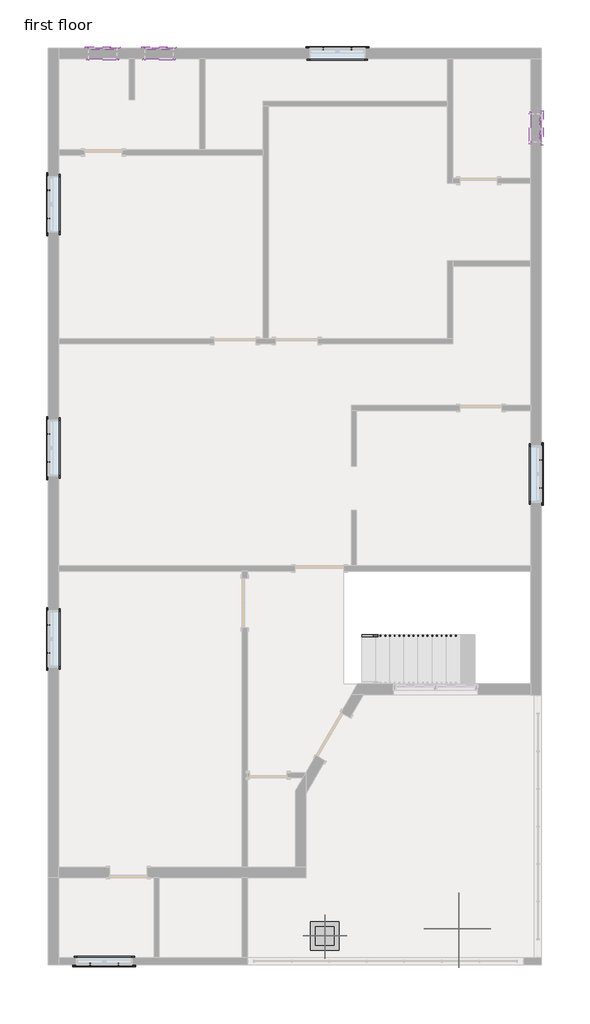
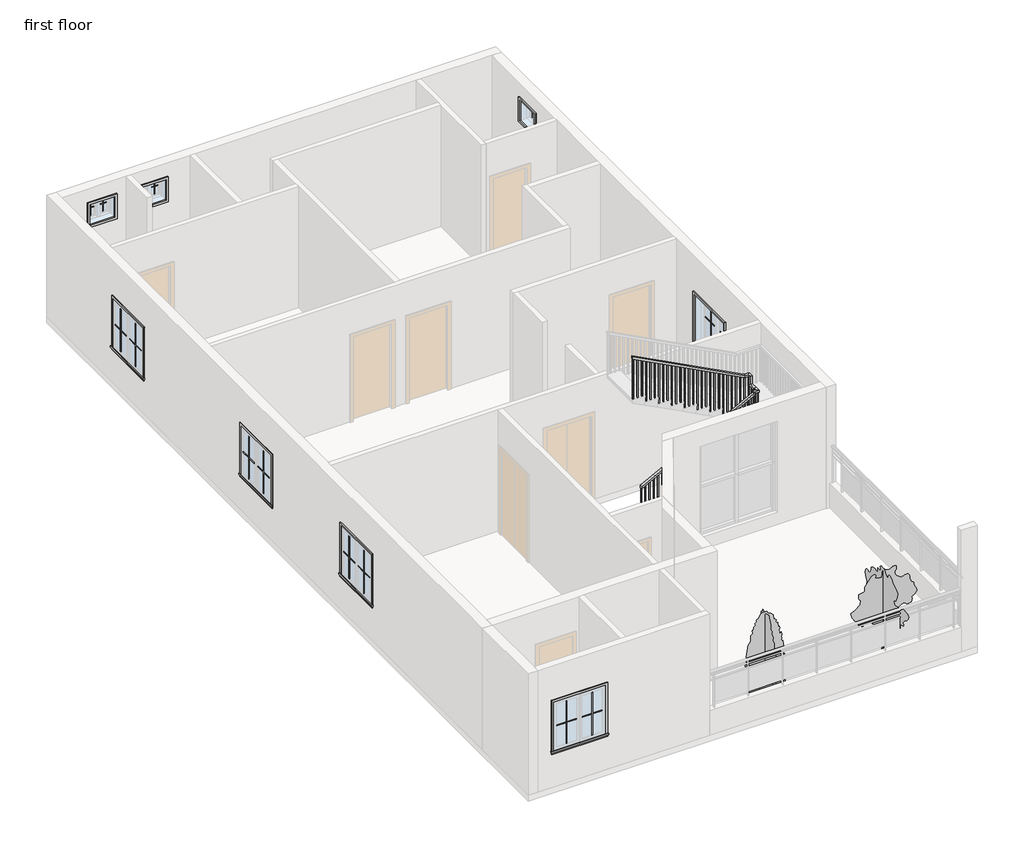
# One storey, part 4 of 4: 36 proxies, 3 geographic elements, 1 railing.
"""IFC4 building model written with IfcOpenShell, lengths in millimetres."""

from ifc_helpers import new_model, si_unit, frame, origin, place, context, project, spatial, polyline, outline, extrude, faceted_brep, transform, mapped, element, save
from components import muntin_pattern_2x2_muntin_pattern_2x2_4dfeb3f3, muntin_pattern_2x2_muntin_pattern_2x2_e852a7e4, muntin_pattern_2x2_muntin_pattern_2x2_653c8599, muntin_pattern_2x2_muntin_pattern_2x2_c179cf80, trim_window_exterior_flat_with_sill_7cfdd449, trim_window_exterior_flat_with_sill_e6f34eb5, trim_window_interior_flat_picture_frame_f1e0b15b, trim_window_interior_flat_picture_frame_9a74d23d, planter_2_x2_da431093, rpc_tree_conifer_chinese_juniper_7_1b9786cd, rpc_tree_deciduous_japanese_cherry_15_720dba75

model = new_model("IFC4")

# Units and contexts
model_context = context("Model", 3, world=origin())
ifc_project = project(units=[si_unit("LENGTHUNIT", "METRE", prefix="MILLI")], contexts=[model_context])

# Site, building, storey
site = spatial("IfcSite", under=ifc_project)
building = spatial("IfcBuilding", under=site)
storey = spatial("IfcBuildingStorey", under=building, Name="first floor", Elevation=3200.4)

# Proxies
placement = place(None, origin())
muntin_pattern_2x2_muntin_pattern_2x2_shape = muntin_pattern_2x2_muntin_pattern_2x2_4dfeb3f3(model_context)
element("IfcBuildingElementProxy", 1, Name="Muntin Pattern_2x2 : Muntin Pattern_2x2", ObjectType="Muntin Pattern_2x2 : Muntin Pattern_2x2", at=placement, inside=storey, context=model_context, shape_type="MappedRepresentation", body=[
    mapped(muntin_pattern_2x2_muntin_pattern_2x2_shape, transform((-5762.6039904, 6482.7851094, 4184.65), x_axis=(0.0, 1.0, 0.0), y_axis=(-1.0, 0.0, 0.0), z_axis=(0.0, 0.0, 1.0))),
])
element("IfcBuildingElementProxy", 2, Name="Muntin Pattern_2x2 : Muntin Pattern_2x2", ObjectType="Muntin Pattern_2x2 : Muntin Pattern_2x2", at=placement, inside=storey, context=model_context, shape_type="MappedRepresentation", body=[
    mapped(muntin_pattern_2x2_muntin_pattern_2x2_shape, transform((-5762.6039904, 1212.2851094, 4184.65), x_axis=(0.0, 1.0, 0.0), y_axis=(-1.0, 0.0, 0.0), z_axis=(0.0, 0.0, 1.0))),
])
element("IfcBuildingElementProxy", 3, Name="Muntin Pattern_2x2 : Muntin Pattern_2x2", ObjectType="Muntin Pattern_2x2 : Muntin Pattern_2x2", at=placement, inside=storey, context=model_context, shape_type="MappedRepresentation", body=[
    mapped(muntin_pattern_2x2_muntin_pattern_2x2_shape, transform((-5762.6039904, -2915.2148906, 4184.65), x_axis=(0.0, 1.0, 0.0), y_axis=(-1.0, 0.0, 0.0), z_axis=(0.0, 0.0, 1.0))),
])
element("IfcBuildingElementProxy", 4, Name="Muntin Pattern_2x2 : Muntin Pattern_2x2", ObjectType="Muntin Pattern_2x2 : Muntin Pattern_2x2", at=placement, inside=storey, context=model_context, shape_type="MappedRepresentation", body=[
    mapped(muntin_pattern_2x2_muntin_pattern_2x2_shape, transform((4887.9335096, 1259.9101094, 4184.65), x_axis=(0.0, -1.0, 0.0), y_axis=(1.0, 0.0, 0.0), z_axis=(0.0, 0.0, 1.0))),
])
element("IfcBuildingElementProxy", 5, Name="Muntin Pattern_2x2 : Muntin Pattern_2x2", ObjectType="Muntin Pattern_2x2 : Muntin Pattern_2x2", at=placement, inside=storey, context=model_context, shape_type="MappedRepresentation", body=[
    mapped(muntin_pattern_2x2_muntin_pattern_2x2_shape, transform((-4258.4477404, -9644.6273906, 4184.65), x_axis=(-1.0, 0.0, 0.0), y_axis=(0.0, -1.0, 0.0), z_axis=(0.0, 0.0, 1.0))),
])
element("IfcBuildingElementProxy", 6, Name="Muntin Pattern_2x2 : Muntin Pattern_2x2", ObjectType="Muntin Pattern_2x2 : Muntin Pattern_2x2", at=placement, inside=storey, context=model_context, shape_type="MappedRepresentation", body=[
    mapped(muntin_pattern_2x2_muntin_pattern_2x2_shape, transform((180.9960096, 10148.3226094, 4184.65), x_axis=(1.0, 0.0, 0.0), y_axis=(0.0, 1.0, 0.0), z_axis=(0.0, 0.0, 1.0))),
])
muntin_pattern_2x2_muntin_pattern_2x2_2_shape = muntin_pattern_2x2_muntin_pattern_2x2_e852a7e4(model_context)
element("IfcBuildingElementProxy", 7, Name="Muntin Pattern_2x2 : Muntin Pattern_2x2", ObjectType="Muntin Pattern_2x2 : Muntin Pattern_2x2", at=placement, inside=storey, context=model_context, shape_type="MappedRepresentation", body=[
    mapped(muntin_pattern_2x2_muntin_pattern_2x2_2_shape, transform((-5762.6039904, 7089.2101094, 4184.65), x_axis=(0.0, -1.0, 0.0), y_axis=(1.0, 0.0, 0.0), z_axis=(0.0, 0.0, 1.0))),
])
element("IfcBuildingElementProxy", 8, Name="Muntin Pattern_2x2 : Muntin Pattern_2x2", ObjectType="Muntin Pattern_2x2 : Muntin Pattern_2x2", at=placement, inside=storey, context=model_context, shape_type="MappedRepresentation", body=[
    mapped(muntin_pattern_2x2_muntin_pattern_2x2_2_shape, transform((-5762.6039904, 1818.7101094, 4184.65), x_axis=(0.0, -1.0, 0.0), y_axis=(1.0, 0.0, 0.0), z_axis=(0.0, 0.0, 1.0))),
])
element("IfcBuildingElementProxy", 9, Name="Muntin Pattern_2x2 : Muntin Pattern_2x2", ObjectType="Muntin Pattern_2x2 : Muntin Pattern_2x2", at=placement, inside=storey, context=model_context, shape_type="MappedRepresentation", body=[
    mapped(muntin_pattern_2x2_muntin_pattern_2x2_2_shape, transform((-5762.6039904, -2308.7898906, 4184.65), x_axis=(0.0, -1.0, 0.0), y_axis=(1.0, 0.0, 0.0), z_axis=(0.0, 0.0, 1.0))),
])
element("IfcBuildingElementProxy", 10, Name="Muntin Pattern_2x2 : Muntin Pattern_2x2", ObjectType="Muntin Pattern_2x2 : Muntin Pattern_2x2", at=placement, inside=storey, context=model_context, shape_type="MappedRepresentation", body=[
    mapped(muntin_pattern_2x2_muntin_pattern_2x2_2_shape, transform((4887.9335096, 653.4851094, 4184.65), x_axis=(0.0, 1.0, 0.0), y_axis=(-1.0, 0.0, 0.0), z_axis=(0.0, 0.0, 1.0))),
])
element("IfcBuildingElementProxy", 11, Name="Muntin Pattern_2x2 : Muntin Pattern_2x2", ObjectType="Muntin Pattern_2x2 : Muntin Pattern_2x2", at=placement, inside=storey, context=model_context, shape_type="MappedRepresentation", body=[
    mapped(muntin_pattern_2x2_muntin_pattern_2x2_2_shape, transform((-4864.8727404, -9644.6273906, 4184.65), x_axis=(1.0, 0.0, 0.0), y_axis=(0.0, 1.0, 0.0), z_axis=(0.0, 0.0, 1.0))),
])
element("IfcBuildingElementProxy", 12, Name="Muntin Pattern_2x2 : Muntin Pattern_2x2", ObjectType="Muntin Pattern_2x2 : Muntin Pattern_2x2", at=placement, inside=storey, context=model_context, shape_type="MappedRepresentation", body=[
    mapped(muntin_pattern_2x2_muntin_pattern_2x2_2_shape, transform((787.4210096, 10148.3226094, 4184.65), x_axis=(-1.0, 0.0, 0.0), y_axis=(0.0, -1.0, 0.0), z_axis=(0.0, 0.0, 1.0))),
])
muntin_pattern_2x2_muntin_pattern_2x2_3_shape = muntin_pattern_2x2_muntin_pattern_2x2_653c8599(model_context)
element("IfcBuildingElementProxy", 13, Name="Muntin Pattern_2x2 : Muntin Pattern_2x2", ObjectType="Muntin Pattern_2x2 : Muntin Pattern_2x2", at=placement, inside=storey, context=model_context, shape_type="MappedRepresentation", body=[
    mapped(muntin_pattern_2x2_muntin_pattern_2x2_3_shape, transform((-4746.6039904, 10148.3226094, 5403.85), x_axis=(1.0, 0.0, 0.0), y_axis=(0.0, 1.0, 0.0), z_axis=(0.0, 0.0, 1.0))),
])
element("IfcBuildingElementProxy", 14, Name="Muntin Pattern_2x2 : Muntin Pattern_2x2", ObjectType="Muntin Pattern_2x2 : Muntin Pattern_2x2", at=placement, inside=storey, context=model_context, shape_type="MappedRepresentation", body=[
    mapped(muntin_pattern_2x2_muntin_pattern_2x2_3_shape, transform((-3527.4039904, 10148.3226094, 5403.85), x_axis=(1.0, 0.0, 0.0), y_axis=(0.0, 1.0, 0.0), z_axis=(0.0, 0.0, 1.0))),
])
element("IfcBuildingElementProxy", 15, Name="Muntin Pattern_2x2 : Muntin Pattern_2x2", ObjectType="Muntin Pattern_2x2 : Muntin Pattern_2x2", at=placement, inside=storey, context=model_context, shape_type="MappedRepresentation", body=[
    mapped(muntin_pattern_2x2_muntin_pattern_2x2_3_shape, transform((4887.9335096, 8587.8101094, 5403.85), x_axis=(0.0, -1.0, 0.0), y_axis=(1.0, 0.0, 0.0), z_axis=(0.0, 0.0, 1.0))),
])
muntin_pattern_2x2_muntin_pattern_2x2_4_shape = muntin_pattern_2x2_muntin_pattern_2x2_c179cf80(model_context)
element("IfcBuildingElementProxy", 16, Name="Muntin Pattern_2x2 : Muntin Pattern_2x2", ObjectType="Muntin Pattern_2x2 : Muntin Pattern_2x2", at=placement, inside=storey, context=model_context, shape_type="MappedRepresentation", body=[
    mapped(muntin_pattern_2x2_muntin_pattern_2x2_4_shape, transform((-4444.9789904, 10148.3226094, 5403.85), x_axis=(-1.0, 0.0, 0.0), y_axis=(0.0, -1.0, 0.0), z_axis=(0.0, 0.0, 1.0))),
])
element("IfcBuildingElementProxy", 17, Name="Muntin Pattern_2x2 : Muntin Pattern_2x2", ObjectType="Muntin Pattern_2x2 : Muntin Pattern_2x2", at=placement, inside=storey, context=model_context, shape_type="MappedRepresentation", body=[
    mapped(muntin_pattern_2x2_muntin_pattern_2x2_4_shape, transform((-3225.7789904, 10148.3226094, 5403.85), x_axis=(-1.0, 0.0, 0.0), y_axis=(0.0, -1.0, 0.0), z_axis=(0.0, 0.0, 1.0))),
])
element("IfcBuildingElementProxy", 18, Name="Muntin Pattern_2x2 : Muntin Pattern_2x2", ObjectType="Muntin Pattern_2x2 : Muntin Pattern_2x2", at=placement, inside=storey, context=model_context, shape_type="MappedRepresentation", body=[
    mapped(muntin_pattern_2x2_muntin_pattern_2x2_4_shape, transform((4887.9335096, 8286.1851094, 5403.85), x_axis=(0.0, 1.0, 0.0), y_axis=(-1.0, 0.0, 0.0), z_axis=(0.0, 0.0, 1.0))),
])
trim_window_exterior_flat_with_sill_shape = trim_window_exterior_flat_with_sill_7cfdd449(model_context)
element("IfcBuildingElementProxy", 19, Name="Trim-Window-Exterior-Flat : with Sill", ObjectType="Trim-Window-Exterior-Flat : with Sill", at=placement, inside=storey, context=model_context, shape_type="MappedRepresentation", body=[
    mapped(trim_window_exterior_flat_with_sill_shape, transform((-5772.1289904, 6785.9976094, 5334.0), x_axis=(0.0, -1.0, 0.0), y_axis=(0.0, 0.0, 1.0), z_axis=(-1.0, 0.0, 0.0))),
])
element("IfcBuildingElementProxy", 20, Name="Trim-Window-Exterior-Flat : with Sill", ObjectType="Trim-Window-Exterior-Flat : with Sill", at=placement, inside=storey, context=model_context, shape_type="MappedRepresentation", body=[
    mapped(trim_window_exterior_flat_with_sill_shape, transform((-5772.1289904, 1515.4976094, 5334.0), x_axis=(0.0, -1.0, 0.0), y_axis=(0.0, 0.0, 1.0), z_axis=(-1.0, 0.0, 0.0))),
])
element("IfcBuildingElementProxy", 21, Name="Trim-Window-Exterior-Flat : with Sill", ObjectType="Trim-Window-Exterior-Flat : with Sill", at=placement, inside=storey, context=model_context, shape_type="MappedRepresentation", body=[
    mapped(trim_window_exterior_flat_with_sill_shape, transform((-5772.1289904, -2612.0023906, 5334.0), x_axis=(0.0, -1.0, 0.0), y_axis=(0.0, 0.0, 1.0), z_axis=(-1.0, 0.0, 0.0))),
])
element("IfcBuildingElementProxy", 22, Name="Trim-Window-Exterior-Flat : with Sill", ObjectType="Trim-Window-Exterior-Flat : with Sill", at=placement, inside=storey, context=model_context, shape_type="MappedRepresentation", body=[
    mapped(trim_window_exterior_flat_with_sill_shape, transform((4897.4585096, 956.6976094, 5334.0), x_axis=(0.0, 1.0, 0.0), y_axis=(0.0, 0.0, 1.0), z_axis=(1.0, 0.0, 0.0))),
])
element("IfcBuildingElementProxy", 23, Name="Trim-Window-Exterior-Flat : with Sill", ObjectType="Trim-Window-Exterior-Flat : with Sill", at=placement, inside=storey, context=model_context, shape_type="MappedRepresentation", body=[
    mapped(trim_window_exterior_flat_with_sill_shape, transform((-4561.6602404, -9654.1523906, 5334.0), x_axis=(1.0, 0.0, 0.0), y_axis=(0.0, 0.0, 1.0), z_axis=(0.0, -1.0, 0.0))),
])
element("IfcBuildingElementProxy", 24, Name="Trim-Window-Exterior-Flat : with Sill", ObjectType="Trim-Window-Exterior-Flat : with Sill", at=placement, inside=storey, context=model_context, shape_type="MappedRepresentation", body=[
    mapped(trim_window_exterior_flat_with_sill_shape, transform((484.2085096, 10157.8476094, 5334.0), x_axis=(-1.0, 0.0, 0.0), y_axis=(0.0, 0.0, 1.0), z_axis=(0.0, 1.0, 0.0))),
])
trim_window_exterior_flat_with_sill_2_shape = trim_window_exterior_flat_with_sill_e6f34eb5(model_context)
element("IfcBuildingElementProxy", 25, Name="Trim-Window-Exterior-Flat : with Sill", ObjectType="Trim-Window-Exterior-Flat : with Sill", at=placement, inside=storey, context=model_context, shape_type="MappedRepresentation", body=[
    mapped(trim_window_exterior_flat_with_sill_2_shape, transform((-4595.7914904, 10157.8476094, 5867.4), x_axis=(-1.0, 0.0, 0.0), y_axis=(0.0, 0.0, 1.0), z_axis=(0.0, 1.0, 0.0))),
])
element("IfcBuildingElementProxy", 26, Name="Trim-Window-Exterior-Flat : with Sill", ObjectType="Trim-Window-Exterior-Flat : with Sill", at=placement, inside=storey, context=model_context, shape_type="MappedRepresentation", body=[
    mapped(trim_window_exterior_flat_with_sill_2_shape, transform((-3376.5914904, 10157.8476094, 5867.4), x_axis=(-1.0, 0.0, 0.0), y_axis=(0.0, 0.0, 1.0), z_axis=(0.0, 1.0, 0.0))),
])
element("IfcBuildingElementProxy", 27, Name="Trim-Window-Exterior-Flat : with Sill", ObjectType="Trim-Window-Exterior-Flat : with Sill", at=placement, inside=storey, context=model_context, shape_type="MappedRepresentation", body=[
    mapped(trim_window_exterior_flat_with_sill_2_shape, transform((4897.4585096, 8436.9976094, 5867.4), x_axis=(0.0, 1.0, 0.0), y_axis=(0.0, 0.0, 1.0), z_axis=(1.0, 0.0, 0.0))),
])
trim_window_interior_flat_picture_frame_shape = trim_window_interior_flat_picture_frame_f1e0b15b(model_context)
element("IfcBuildingElementProxy", 28, Name="Trim-Window-Interior-Flat : Picture Frame", ObjectType="Trim-Window-Interior-Flat : Picture Frame", at=placement, inside=storey, context=model_context, shape_type="MappedRepresentation", body=[
    mapped(trim_window_interior_flat_picture_frame_shape, transform((-5543.5289904, 6785.9976094, 5334.0), x_axis=(0.0, 1.0, 0.0), y_axis=(0.0, 0.0, 1.0), z_axis=(1.0, 0.0, 0.0))),
])
element("IfcBuildingElementProxy", 29, Name="Trim-Window-Interior-Flat : Picture Frame", ObjectType="Trim-Window-Interior-Flat : Picture Frame", at=placement, inside=storey, context=model_context, shape_type="MappedRepresentation", body=[
    mapped(trim_window_interior_flat_picture_frame_shape, transform((-5543.5289904, 1515.4976094, 5334.0), x_axis=(0.0, 1.0, 0.0), y_axis=(0.0, 0.0, 1.0), z_axis=(1.0, 0.0, 0.0))),
])
element("IfcBuildingElementProxy", 30, Name="Trim-Window-Interior-Flat : Picture Frame", ObjectType="Trim-Window-Interior-Flat : Picture Frame", at=placement, inside=storey, context=model_context, shape_type="MappedRepresentation", body=[
    mapped(trim_window_interior_flat_picture_frame_shape, transform((-5543.5289904, -2612.0023906, 5334.0), x_axis=(0.0, 1.0, 0.0), y_axis=(0.0, 0.0, 1.0), z_axis=(1.0, 0.0, 0.0))),
])
element("IfcBuildingElementProxy", 31, Name="Trim-Window-Interior-Flat : Picture Frame", ObjectType="Trim-Window-Interior-Flat : Picture Frame", at=placement, inside=storey, context=model_context, shape_type="MappedRepresentation", body=[
    mapped(trim_window_interior_flat_picture_frame_shape, transform((4668.8585096, 956.6976094, 5334.0), x_axis=(0.0, -1.0, 0.0), y_axis=(0.0, 0.0, 1.0), z_axis=(-1.0, 0.0, 0.0))),
])
element("IfcBuildingElementProxy", 32, Name="Trim-Window-Interior-Flat : Picture Frame", ObjectType="Trim-Window-Interior-Flat : Picture Frame", at=placement, inside=storey, context=model_context, shape_type="MappedRepresentation", body=[
    mapped(trim_window_interior_flat_picture_frame_shape, transform((-4561.6602404, -9501.7523906, 5334.0), x_axis=(-1.0, 0.0, 0.0), y_axis=(0.0, 0.0, 1.0), z_axis=(0.0, 1.0, 0.0))),
])
element("IfcBuildingElementProxy", 33, Name="Trim-Window-Interior-Flat : Picture Frame", ObjectType="Trim-Window-Interior-Flat : Picture Frame", at=placement, inside=storey, context=model_context, shape_type="MappedRepresentation", body=[
    mapped(trim_window_interior_flat_picture_frame_shape, transform((484.2085096, 9929.2476094, 5334.0), x_axis=(1.0, 0.0, 0.0), y_axis=(0.0, 0.0, 1.0), z_axis=(0.0, -1.0, 0.0))),
])
trim_window_interior_flat_picture_frame_2_shape = trim_window_interior_flat_picture_frame_9a74d23d(model_context)
element("IfcBuildingElementProxy", 34, Name="Trim-Window-Interior-Flat : Picture Frame", ObjectType="Trim-Window-Interior-Flat : Picture Frame", at=placement, inside=storey, context=model_context, shape_type="MappedRepresentation", body=[
    mapped(trim_window_interior_flat_picture_frame_2_shape, transform((-4595.7914904, 9929.2476094, 5867.4), x_axis=(1.0, 0.0, 0.0), y_axis=(0.0, 0.0, 1.0), z_axis=(0.0, -1.0, 0.0))),
])
element("IfcBuildingElementProxy", 35, Name="Trim-Window-Interior-Flat : Picture Frame", ObjectType="Trim-Window-Interior-Flat : Picture Frame", at=placement, inside=storey, context=model_context, shape_type="MappedRepresentation", body=[
    mapped(trim_window_interior_flat_picture_frame_2_shape, transform((-3376.5914904, 9929.2476094, 5867.4), x_axis=(1.0, 0.0, 0.0), y_axis=(0.0, 0.0, 1.0), z_axis=(0.0, -1.0, 0.0))),
])
element("IfcBuildingElementProxy", 36, Name="Trim-Window-Interior-Flat : Picture Frame", ObjectType="Trim-Window-Interior-Flat : Picture Frame", at=placement, inside=storey, context=model_context, shape_type="MappedRepresentation", body=[
    mapped(trim_window_interior_flat_picture_frame_2_shape, transform((4668.8585096, 8436.9976094, 5867.4), x_axis=(0.0, -1.0, 0.0), y_axis=(0.0, 0.0, 1.0), z_axis=(-1.0, 0.0, 0.0))),
])

# Geographic elements
planter_2_x2_shape = planter_2_x2_da431093(model_context)
element("IfcGeographicElement", 37, ObjectType="Planter : 2'x2'", at=placement, inside=storey, context=model_context, shape_type="MappedRepresentation", body=[
    mapped(planter_2_x2_shape, transform((211.1585096, -9031.8523906, 3200.4), x_axis=(1.0, 0.0, 0.0), y_axis=(0.0, 1.0, 0.0), z_axis=(0.0, 0.0, 1.0))),
])
rpc_tree_conifer_chinese_juniper_7_shape = rpc_tree_conifer_chinese_juniper_7_1b9786cd(model_context)
element("IfcGeographicElement", 38, ObjectType="RPC Tree - Conifer : Chinese Juniper - 7'", at=placement, inside=storey, context=model_context, shape_type="MappedRepresentation", body=[
    mapped(rpc_tree_conifer_chinese_juniper_7_shape, transform((210.9618385, -9031.8523906, 3200.4), x_axis=(1.0, 0.0, 0.0), y_axis=(0.0, 1.0, 0.0), z_axis=(0.0, 0.0, 1.0))),
])
rpc_tree_deciduous_japanese_cherry_15_shape = rpc_tree_deciduous_japanese_cherry_15_720dba75(model_context)
element("IfcGeographicElement", 39, ObjectType="RPC Tree - Deciduous : Japanese Cherry - 15'", at=placement, inside=storey, context=model_context, shape_type="MappedRepresentation", body=[
    mapped(rpc_tree_deciduous_japanese_cherry_15_shape, transform((3106.7585096, -8879.4523906, 3200.4), x_axis=(1.0, 0.0, 0.0), y_axis=(0.0, 1.0, 0.0), z_axis=(0.0, 0.0, 1.0))),
])

# Railing
element("IfcRailing", 40, ObjectType="Handrail - Rectangular", at=placement, inside=storey, context=model_context, shape_type="SolidModel", body=[
    faceted_brep([(1011.2585096, -2516.7523906, 4274.82), (1011.2585096, -2516.7523906, 4217.4446664), (1011.2585096, -2567.5523906, 4217.4446664), (1011.2585096, -2567.5523906, 4274.82), (3678.2585096, -2516.7523906, 5674.995), (3729.0585096, -2516.7523906, 5644.2896664), (3729.0585096, -2567.5523906, 5644.2896664), (3678.2585096, -2567.5523906, 5674.995), (3678.2585096, -2516.7523906, 5715.0), (3729.0585096, -2516.7523906, 5664.2), (3729.0585096, -2567.5523906, 5664.2), (3678.2585096, -2567.5523906, 5715.0), (3754.4585096, -2516.7523906, 5715.0), (3754.4585096, -2516.7523906, 5664.2), (3805.2585096, -2567.5523906, 5664.2), (3805.2585096, -2567.5523906, 5715.0), (3754.4585096, -2440.5523906, 5715.0), (3754.4585096, -2440.5523906, 5664.2), (3805.2585096, -2440.5523906, 5664.2), (3805.2585096, -2440.5523906, 5715.0), (3754.4585096, -2288.1523906, 5715.0), (3754.4585096, -2237.3523906, 5664.2), (3805.2585096, -2237.3523906, 5664.2), (3805.2585096, -2288.1523906, 5715.0), (3754.4585096, -2288.1523906, 5915.025), (3754.4585096, -2237.3523906, 5864.225), (3805.2585096, -2237.3523906, 5864.225), (3805.2585096, -2288.1523906, 5915.025), (3754.4585096, -2211.9523906, 5915.025), (3754.4585096, -2211.9523906, 5864.225), (3805.2585096, -2161.1523906, 5864.225), (3805.2585096, -2161.1523906, 5915.025), (3678.2585096, -2211.9523906, 5915.025), (3665.7340647, -2211.9523906, 5864.225), (3665.7340647, -2161.1523906, 5864.225), (3678.2585096, -2161.1523906, 5915.025), (1011.2585096, -2211.9523906, 7315.2), (1011.2585096, -2161.1523906, 7315.2), (1011.2585096, -2161.1523906, 7257.8246664), (1011.2585096, -2211.9523906, 7257.8246664)], [[[0, 1, 2, 3]], [[1, 0, 4, 5]], [[2, 1, 5, 6]], [[3, 2, 6, 7]], [[0, 3, 7, 4]], [[5, 4, 8, 9]], [[6, 5, 9, 10]], [[7, 6, 10, 11]], [[4, 7, 11, 8]], [[9, 8, 12, 13]], [[10, 9, 13, 14]], [[11, 10, 14, 15]], [[8, 11, 15, 12]], [[13, 12, 16, 17]], [[14, 13, 17, 18]], [[15, 14, 18, 19]], [[12, 15, 19, 16]], [[17, 16, 20, 21]], [[18, 17, 21, 22]], [[19, 18, 22, 23]], [[16, 19, 23, 20]], [[21, 20, 24, 25]], [[22, 21, 25, 26]], [[23, 22, 26, 27]], [[20, 23, 27, 24]], [[25, 24, 28, 29]], [[26, 25, 29, 30]], [[27, 26, 30, 31]], [[24, 27, 31, 28]], [[29, 28, 32, 33]], [[30, 29, 33, 34]], [[31, 30, 34, 35]], [[28, 31, 35, 32]], [[36, 37, 38, 39]], [[33, 32, 36, 39]], [[34, 33, 39, 38]], [[35, 34, 38, 37]], [[32, 35, 37, 36]]]),
    extrude(outline(polyline([(7249.4902914, 1027.1335096), (6240.78, 1027.1335096), (6240.78, 1046.1835096), (7239.4890414, 1046.1835096), (7249.4902914, 1027.1335096)])), frame((0.0, -2196.0773906, 0.0), z_axis=(0.0, 1.0, 0.0), x_axis=(0.0, 0.0, 1.0)), (0.0, 0.0, 1.0), 19.05),
    extrude(outline(polyline([(7196.1502914, 1128.7335096), (6240.78, 1128.7335096), (6240.78, 1147.7835096), (7186.1490414, 1147.7835096), (7196.1502914, 1128.7335096)])), frame((0.0, -2196.0773906, 0.0), z_axis=(0.0, 1.0, 0.0), x_axis=(0.0, 0.0, 1.0)), (0.0, 0.0, 1.0), 19.05),
    extrude(outline(polyline([(7142.8102914, 1230.3335096), (6240.78, 1230.3335096), (6240.78, 1249.3835096), (7132.8090414, 1249.3835096), (7142.8102914, 1230.3335096)])), frame((0.0, -2196.0773906, 0.0), z_axis=(0.0, 1.0, 0.0), x_axis=(0.0, 0.0, 1.0)), (0.0, 0.0, 1.0), 19.05),
    extrude(outline(polyline([(7089.4702914, 1331.9335096), (6080.76, 1331.9335096), (6080.76, 1350.9835096), (7079.4690414, 1350.9835096), (7089.4702914, 1331.9335096)])), frame((0.0, -2196.0773906, 0.0), z_axis=(0.0, 1.0, 0.0), x_axis=(0.0, 0.0, 1.0)), (0.0, 0.0, 1.0), 19.05),
    extrude(outline(polyline([(7036.1302914, 1433.5335096), (6080.76, 1433.5335096), (6080.76, 1452.5835096), (7026.1290414, 1452.5835096), (7036.1302914, 1433.5335096)])), frame((0.0, -2196.0773906, 0.0), z_axis=(0.0, 1.0, 0.0), x_axis=(0.0, 0.0, 1.0)), (0.0, 0.0, 1.0), 19.05),
    extrude(outline(polyline([(6982.7902914, 1535.1335096), (6080.76, 1535.1335096), (6080.76, 1554.1835096), (6972.7890414, 1554.1835096), (6982.7902914, 1535.1335096)])), frame((0.0, -2196.0773906, 0.0), z_axis=(0.0, 1.0, 0.0), x_axis=(0.0, 0.0, 1.0)), (0.0, 0.0, 1.0), 19.05),
    extrude(outline(polyline([(6929.4502914, 1636.7335096), (5920.74, 1636.7335096), (5920.74, 1655.7835096), (6919.4490414, 1655.7835096), (6929.4502914, 1636.7335096)])), frame((0.0, -2196.0773906, 0.0), z_axis=(0.0, 1.0, 0.0), x_axis=(0.0, 0.0, 1.0)), (0.0, 0.0, 1.0), 19.05),
    extrude(outline(polyline([(6876.1102914, 1738.3335096), (5920.74, 1738.3335096), (5920.74, 1757.3835096), (6866.1090414, 1757.3835096), (6876.1102914, 1738.3335096)])), frame((0.0, -2196.0773906, 0.0), z_axis=(0.0, 1.0, 0.0), x_axis=(0.0, 0.0, 1.0)), (0.0, 0.0, 1.0), 19.05),
    extrude(outline(polyline([(6822.7702914, 1839.9335096), (5920.74, 1839.9335096), (5920.74, 1858.9835096), (6812.7690414, 1858.9835096), (6822.7702914, 1839.9335096)])), frame((0.0, -2196.0773906, 0.0), z_axis=(0.0, 1.0, 0.0), x_axis=(0.0, 0.0, 1.0)), (0.0, 0.0, 1.0), 19.05),
    extrude(outline(polyline([(6769.4302914, 1941.5335096), (5760.72, 1941.5335096), (5760.72, 1960.5835096), (6759.4290414, 1960.5835096), (6769.4302914, 1941.5335096)])), frame((0.0, -2196.0773906, 0.0), z_axis=(0.0, 1.0, 0.0), x_axis=(0.0, 0.0, 1.0)), (0.0, 0.0, 1.0), 19.05),
    extrude(outline(polyline([(6716.0902914, 2043.1335096), (5760.72, 2043.1335096), (5760.72, 2062.1835096), (6706.0890414, 2062.1835096), (6716.0902914, 2043.1335096)])), frame((0.0, -2196.0773906, 0.0), z_axis=(0.0, 1.0, 0.0), x_axis=(0.0, 0.0, 1.0)), (0.0, 0.0, 1.0), 19.05),
    extrude(outline(polyline([(6662.7502914, 2144.7335096), (5760.72, 2144.7335096), (5760.72, 2163.7835096), (6652.7490414, 2163.7835096), (6662.7502914, 2144.7335096)])), frame((0.0, -2196.0773906, 0.0), z_axis=(0.0, 1.0, 0.0), x_axis=(0.0, 0.0, 1.0)), (0.0, 0.0, 1.0), 19.05),
    extrude(outline(polyline([(6609.4102914, 2246.3335096), (5600.7, 2246.3335096), (5600.7, 2265.3835096), (6599.4090414, 2265.3835096), (6609.4102914, 2246.3335096)])), frame((0.0, -2196.0773906, 0.0), z_axis=(0.0, 1.0, 0.0), x_axis=(0.0, 0.0, 1.0)), (0.0, 0.0, 1.0), 19.05),
    extrude(outline(polyline([(6556.0702914, 2347.9335096), (5600.7, 2347.9335096), (5600.7, 2366.9835096), (6546.0690414, 2366.9835096), (6556.0702914, 2347.9335096)])), frame((0.0, -2196.0773906, 0.0), z_axis=(0.0, 1.0, 0.0), x_axis=(0.0, 0.0, 1.0)), (0.0, 0.0, 1.0), 19.05),
    extrude(outline(polyline([(6502.7302914, 2449.5335096), (5600.7, 2449.5335096), (5600.7, 2468.5835096), (6492.7290414, 2468.5835096), (6502.7302914, 2449.5335096)])), frame((0.0, -2196.0773906, 0.0), z_axis=(0.0, 1.0, 0.0), x_axis=(0.0, 0.0, 1.0)), (0.0, 0.0, 1.0), 19.05),
    extrude(outline(polyline([(6449.3902914, 2551.1335096), (5440.68, 2551.1335096), (5440.68, 2570.1835096), (6439.3890414, 2570.1835096), (6449.3902914, 2551.1335096)])), frame((0.0, -2196.0773906, 0.0), z_axis=(0.0, 1.0, 0.0), x_axis=(0.0, 0.0, 1.0)), (0.0, 0.0, 1.0), 19.05),
    extrude(outline(polyline([(6396.0502914, 2652.7335096), (5440.68, 2652.7335096), (5440.68, 2671.7835096), (6386.0490414, 2671.7835096), (6396.0502914, 2652.7335096)])), frame((0.0, -2196.0773906, 0.0), z_axis=(0.0, 1.0, 0.0), x_axis=(0.0, 0.0, 1.0)), (0.0, 0.0, 1.0), 19.05),
    extrude(outline(polyline([(6342.7102914, 2754.3335096), (5440.68, 2754.3335096), (5440.68, 2773.3835096), (6332.7090414, 2773.3835096), (6342.7102914, 2754.3335096)])), frame((0.0, -2196.0773906, 0.0), z_axis=(0.0, 1.0, 0.0), x_axis=(0.0, 0.0, 1.0)), (0.0, 0.0, 1.0), 19.05),
    extrude(outline(polyline([(6289.3702914, 2855.9335096), (5280.66, 2855.9335096), (5280.66, 2874.9835096), (6279.3690414, 2874.9835096), (6289.3702914, 2855.9335096)])), frame((0.0, -2196.0773906, 0.0), z_axis=(0.0, 1.0, 0.0), x_axis=(0.0, 0.0, 1.0)), (0.0, 0.0, 1.0), 19.05),
    extrude(outline(polyline([(6236.0302914, 2957.5335096), (5280.66, 2957.5335096), (5280.66, 2976.5835096), (6226.0290414, 2976.5835096), (6236.0302914, 2957.5335096)])), frame((0.0, -2196.0773906, 0.0), z_axis=(0.0, 1.0, 0.0), x_axis=(0.0, 0.0, 1.0)), (0.0, 0.0, 1.0), 19.05),
    extrude(outline(polyline([(6182.6902914, 3059.1335096), (5280.66, 3059.1335096), (5280.66, 3078.1835096), (6172.6890414, 3078.1835096), (6182.6902914, 3059.1335096)])), frame((0.0, -2196.0773906, 0.0), z_axis=(0.0, 1.0, 0.0), x_axis=(0.0, 0.0, 1.0)), (0.0, 0.0, 1.0), 19.05),
    extrude(outline(polyline([(6129.3502914, 3160.7335096), (5120.64, 3160.7335096), (5120.64, 3179.7835096), (6119.3490414, 3179.7835096), (6129.3502914, 3160.7335096)])), frame((0.0, -2196.0773906, 0.0), z_axis=(0.0, 1.0, 0.0), x_axis=(0.0, 0.0, 1.0)), (0.0, 0.0, 1.0), 19.05),
    extrude(outline(polyline([(6076.0102914, 3262.3335096), (5120.64, 3262.3335096), (5120.64, 3281.3835096), (6066.0090414, 3281.3835096), (6076.0102914, 3262.3335096)])), frame((0.0, -2196.0773906, 0.0), z_axis=(0.0, 1.0, 0.0), x_axis=(0.0, 0.0, 1.0)), (0.0, 0.0, 1.0), 19.05),
    extrude(outline(polyline([(6022.6702914, 3363.9335096), (5120.64, 3363.9335096), (5120.64, 3382.9835096), (6012.6690414, 3382.9835096), (6022.6702914, 3363.9335096)])), frame((0.0, -2196.0773906, 0.0), z_axis=(0.0, 1.0, 0.0), x_axis=(0.0, 0.0, 1.0)), (0.0, 0.0, 1.0), 19.05),
    extrude(outline(polyline([(5969.3302914, 3465.5335096), (4960.62, 3465.5335096), (4960.62, 3484.5835096), (5959.3290414, 3484.5835096), (5969.3302914, 3465.5335096)])), frame((0.0, -2196.0773906, 0.0), z_axis=(0.0, 1.0, 0.0), x_axis=(0.0, 0.0, 1.0)), (0.0, 0.0, 1.0), 19.05),
    extrude(outline(polyline([(5915.9902914, 3567.1335096), (4960.62, 3567.1335096), (4960.62, 3586.1835096), (5905.9890414, 3586.1835096), (5915.9902914, 3567.1335096)])), frame((0.0, -2196.0773906, 0.0), z_axis=(0.0, 1.0, 0.0), x_axis=(0.0, 0.0, 1.0)), (0.0, 0.0, 1.0), 19.05),
    extrude(outline(polyline([(5862.6502914, 3668.7335096), (4960.62, 3668.7335096), (4960.62, 3687.7835096), (5852.6490414, 3687.7835096), (5862.6502914, 3668.7335096)])), frame((0.0, -2196.0773906, 0.0), z_axis=(0.0, 1.0, 0.0), x_axis=(0.0, 0.0, 1.0)), (0.0, 0.0, 1.0), 19.05),
    extrude(outline(polyline([(3770.3335096, -2246.8773906), (3770.3335096, -2227.8273906), (3789.3835096, -2227.8273906), (3789.3835096, -2246.8773906), (3770.3335096, -2246.8773906)])), frame((0.0, 0.0, 4800.6), z_axis=(0.0, 0.0, 1.0), x_axis=(1.0, 0.0, 0.0)), (0.0, 0.0, 1.0), 1063.625),
    extrude(outline(polyline([(3770.3335096, -2348.4773906), (3770.3335096, -2329.4273906), (3789.3835096, -2329.4273906), (3789.3835096, -2348.4773906), (3770.3335096, -2348.4773906)])), frame((0.0, 0.0, 4800.6), z_axis=(0.0, 0.0, 1.0), x_axis=(1.0, 0.0, 0.0)), (0.0, 0.0, 1.0), 863.6),
    extrude(outline(polyline([(3770.3335096, -2450.0773906), (3770.3335096, -2431.0273906), (3789.3835096, -2431.0273906), (3789.3835096, -2450.0773906), (3770.3335096, -2450.0773906)])), frame((0.0, 0.0, 4800.6), z_axis=(0.0, 0.0, 1.0), x_axis=(1.0, 0.0, 0.0)), (0.0, 0.0, 1.0), 863.6),
    extrude(outline(polyline([(3744.9335096, -2532.6273906), (3763.9835096, -2532.6273906), (3763.9835096, -2551.6773906), (3744.9335096, -2551.6773906), (3744.9335096, -2532.6273906)])), frame((0.0, 0.0, 4800.6), z_axis=(0.0, 0.0, 1.0), x_axis=(1.0, 0.0, 0.0)), (0.0, 0.0, 1.0), 863.6),
    extrude(outline(polyline([(5599.2840414, 3643.3335096), (4640.58, 3643.3335096), (4640.58, 3662.3835096), (5609.2852914, 3662.3835096), (5599.2840414, 3643.3335096)])), frame((0.0, -2551.6773906, 0.0), z_axis=(0.0, 1.0, 0.0), x_axis=(0.0, 0.0, 1.0)), (0.0, 0.0, 1.0), 19.05),
    extrude(outline(polyline([(5545.9440414, 3541.7335096), (4640.58, 3541.7335096), (4640.58, 3560.7835096), (5555.9452914, 3560.7835096), (5545.9440414, 3541.7335096)])), frame((0.0, -2551.6773906, 0.0), z_axis=(0.0, 1.0, 0.0), x_axis=(0.0, 0.0, 1.0)), (0.0, 0.0, 1.0), 19.05),
    extrude(outline(polyline([(5492.6040414, 3440.1335096), (4640.58, 3440.1335096), (4640.58, 3459.1835096), (5502.6052914, 3459.1835096), (5492.6040414, 3440.1335096)])), frame((0.0, -2551.6773906, 0.0), z_axis=(0.0, 1.0, 0.0), x_axis=(0.0, 0.0, 1.0)), (0.0, 0.0, 1.0), 19.05),
    extrude(outline(polyline([(5439.2640414, 3338.5335096), (4480.56, 3338.5335096), (4480.56, 3357.5835096), (5449.2652914, 3357.5835096), (5439.2640414, 3338.5335096)])), frame((0.0, -2551.6773906, 0.0), z_axis=(0.0, 1.0, 0.0), x_axis=(0.0, 0.0, 1.0)), (0.0, 0.0, 1.0), 19.05),
    extrude(outline(polyline([(5385.9240414, 3236.9335096), (4480.56, 3236.9335096), (4480.56, 3255.9835096), (5395.9252914, 3255.9835096), (5385.9240414, 3236.9335096)])), frame((0.0, -2551.6773906, 0.0), z_axis=(0.0, 1.0, 0.0), x_axis=(0.0, 0.0, 1.0)), (0.0, 0.0, 1.0), 19.05),
    extrude(outline(polyline([(5332.5840414, 3135.3335096), (4480.56, 3135.3335096), (4480.56, 3154.3835096), (5342.5852914, 3154.3835096), (5332.5840414, 3135.3335096)])), frame((0.0, -2551.6773906, 0.0), z_axis=(0.0, 1.0, 0.0), x_axis=(0.0, 0.0, 1.0)), (0.0, 0.0, 1.0), 19.05),
    extrude(outline(polyline([(5279.2440414, 3033.7335096), (4320.54, 3033.7335096), (4320.54, 3052.7835096), (5289.2452914, 3052.7835096), (5279.2440414, 3033.7335096)])), frame((0.0, -2551.6773906, 0.0), z_axis=(0.0, 1.0, 0.0), x_axis=(0.0, 0.0, 1.0)), (0.0, 0.0, 1.0), 19.05),
    extrude(outline(polyline([(5225.9040414, 2932.1335096), (4320.54, 2932.1335096), (4320.54, 2951.1835096), (5235.9052914, 2951.1835096), (5225.9040414, 2932.1335096)])), frame((0.0, -2551.6773906, 0.0), z_axis=(0.0, 1.0, 0.0), x_axis=(0.0, 0.0, 1.0)), (0.0, 0.0, 1.0), 19.05),
    extrude(outline(polyline([(5172.5640414, 2830.5335096), (4320.54, 2830.5335096), (4320.54, 2849.5835096), (5182.5652914, 2849.5835096), (5172.5640414, 2830.5335096)])), frame((0.0, -2551.6773906, 0.0), z_axis=(0.0, 1.0, 0.0), x_axis=(0.0, 0.0, 1.0)), (0.0, 0.0, 1.0), 19.05),
    extrude(outline(polyline([(5119.2240414, 2728.9335096), (4160.52, 2728.9335096), (4160.52, 2747.9835096), (5129.2252914, 2747.9835096), (5119.2240414, 2728.9335096)])), frame((0.0, -2551.6773906, 0.0), z_axis=(0.0, 1.0, 0.0), x_axis=(0.0, 0.0, 1.0)), (0.0, 0.0, 1.0), 19.05),
    extrude(outline(polyline([(5065.8840414, 2627.3335096), (4160.52, 2627.3335096), (4160.52, 2646.3835096), (5075.8852914, 2646.3835096), (5065.8840414, 2627.3335096)])), frame((0.0, -2551.6773906, 0.0), z_axis=(0.0, 1.0, 0.0), x_axis=(0.0, 0.0, 1.0)), (0.0, 0.0, 1.0), 19.05),
    extrude(outline(polyline([(5012.5440414, 2525.7335096), (4160.52, 2525.7335096), (4160.52, 2544.7835096), (5022.5452914, 2544.7835096), (5012.5440414, 2525.7335096)])), frame((0.0, -2551.6773906, 0.0), z_axis=(0.0, 1.0, 0.0), x_axis=(0.0, 0.0, 1.0)), (0.0, 0.0, 1.0), 19.05),
    extrude(outline(polyline([(4959.2040414, 2424.1335096), (4000.5, 2424.1335096), (4000.5, 2443.1835096), (4969.2052914, 2443.1835096), (4959.2040414, 2424.1335096)])), frame((0.0, -2551.6773906, 0.0), z_axis=(0.0, 1.0, 0.0), x_axis=(0.0, 0.0, 1.0)), (0.0, 0.0, 1.0), 19.05),
    extrude(outline(polyline([(4905.8640414, 2322.5335096), (4000.5, 2322.5335096), (4000.5, 2341.5835096), (4915.8652914, 2341.5835096), (4905.8640414, 2322.5335096)])), frame((0.0, -2551.6773906, 0.0), z_axis=(0.0, 1.0, 0.0), x_axis=(0.0, 0.0, 1.0)), (0.0, 0.0, 1.0), 19.05),
    extrude(outline(polyline([(4852.5240414, 2220.9335096), (4000.5, 2220.9335096), (4000.5, 2239.9835096), (4862.5252914, 2239.9835096), (4852.5240414, 2220.9335096)])), frame((0.0, -2551.6773906, 0.0), z_axis=(0.0, 1.0, 0.0), x_axis=(0.0, 0.0, 1.0)), (0.0, 0.0, 1.0), 19.05),
    extrude(outline(polyline([(4799.1840414, 2119.3335096), (3840.48, 2119.3335096), (3840.48, 2138.3835096), (4809.1852914, 2138.3835096), (4799.1840414, 2119.3335096)])), frame((0.0, -2551.6773906, 0.0), z_axis=(0.0, 1.0, 0.0), x_axis=(0.0, 0.0, 1.0)), (0.0, 0.0, 1.0), 19.05),
    extrude(outline(polyline([(4745.8440414, 2017.7335096), (3840.48, 2017.7335096), (3840.48, 2036.7835096), (4755.8452914, 2036.7835096), (4745.8440414, 2017.7335096)])), frame((0.0, -2551.6773906, 0.0), z_axis=(0.0, 1.0, 0.0), x_axis=(0.0, 0.0, 1.0)), (0.0, 0.0, 1.0), 19.05),
    extrude(outline(polyline([(4692.5040414, 1916.1335096), (3840.48, 1916.1335096), (3840.48, 1935.1835096), (4702.5052914, 1935.1835096), (4692.5040414, 1916.1335096)])), frame((0.0, -2551.6773906, 0.0), z_axis=(0.0, 1.0, 0.0), x_axis=(0.0, 0.0, 1.0)), (0.0, 0.0, 1.0), 19.05),
    extrude(outline(polyline([(4639.1640414, 1814.5335096), (3680.46, 1814.5335096), (3680.46, 1833.5835096), (4649.1652914, 1833.5835096), (4639.1640414, 1814.5335096)])), frame((0.0, -2551.6773906, 0.0), z_axis=(0.0, 1.0, 0.0), x_axis=(0.0, 0.0, 1.0)), (0.0, 0.0, 1.0), 19.05),
    extrude(outline(polyline([(4585.8240414, 1712.9335096), (3680.46, 1712.9335096), (3680.46, 1731.9835096), (4595.8252914, 1731.9835096), (4585.8240414, 1712.9335096)])), frame((0.0, -2551.6773906, 0.0), z_axis=(0.0, 1.0, 0.0), x_axis=(0.0, 0.0, 1.0)), (0.0, 0.0, 1.0), 19.05),
    extrude(outline(polyline([(4532.4840414, 1611.3335096), (3680.46, 1611.3335096), (3680.46, 1630.3835096), (4542.4852914, 1630.3835096), (4532.4840414, 1611.3335096)])), frame((0.0, -2551.6773906, 0.0), z_axis=(0.0, 1.0, 0.0), x_axis=(0.0, 0.0, 1.0)), (0.0, 0.0, 1.0), 19.05),
    extrude(outline(polyline([(4479.1440414, 1509.7335096), (3520.44, 1509.7335096), (3520.44, 1528.7835096), (4489.1452914, 1528.7835096), (4479.1440414, 1509.7335096)])), frame((0.0, -2551.6773906, 0.0), z_axis=(0.0, 1.0, 0.0), x_axis=(0.0, 0.0, 1.0)), (0.0, 0.0, 1.0), 19.05),
    extrude(outline(polyline([(4425.8040414, 1408.1335096), (3520.44, 1408.1335096), (3520.44, 1427.1835096), (4435.8052914, 1427.1835096), (4425.8040414, 1408.1335096)])), frame((0.0, -2551.6773906, 0.0), z_axis=(0.0, 1.0, 0.0), x_axis=(0.0, 0.0, 1.0)), (0.0, 0.0, 1.0), 19.05),
    extrude(outline(polyline([(4372.4640414, 1306.5335096), (3520.44, 1306.5335096), (3520.44, 1325.5835096), (4382.4652914, 1325.5835096), (4372.4640414, 1306.5335096)])), frame((0.0, -2551.6773906, 0.0), z_axis=(0.0, 1.0, 0.0), x_axis=(0.0, 0.0, 1.0)), (0.0, 0.0, 1.0), 19.05),
    extrude(outline(polyline([(4319.1240414, 1204.9335096), (3360.42, 1204.9335096), (3360.42, 1223.9835096), (4329.1252914, 1223.9835096), (4319.1240414, 1204.9335096)])), frame((0.0, -2551.6773906, 0.0), z_axis=(0.0, 1.0, 0.0), x_axis=(0.0, 0.0, 1.0)), (0.0, 0.0, 1.0), 19.05),
    extrude(outline(polyline([(4265.7840414, 1103.3335096), (3360.42, 1103.3335096), (3360.42, 1122.3835096), (4275.7852914, 1122.3835096), (4265.7840414, 1103.3335096)])), frame((0.0, -2551.6773906, 0.0), z_axis=(0.0, 1.0, 0.0), x_axis=(0.0, 0.0, 1.0)), (0.0, 0.0, 1.0), 19.05),
    extrude(outline(polyline([(3770.3335096, -2196.0773906), (3770.3335096, -2177.0273906), (3789.3835096, -2177.0273906), (3789.3835096, -2196.0773906), (3770.3335096, -2196.0773906)])), frame((0.0, 0.0, 4800.6), z_axis=(0.0, 0.0, 1.0), x_axis=(1.0, 0.0, 0.0)), (0.0, 0.0, 1.0), 1063.625),
    extrude(outline(polyline([(3770.3335096, -2532.6273906), (3789.3835096, -2532.6273906), (3789.3835096, -2551.6773906), (3770.3335096, -2551.6773906), (3770.3335096, -2532.6273906)])), frame((0.0, 0.0, 4800.6), z_axis=(0.0, 0.0, 1.0), x_axis=(1.0, 0.0, 0.0)), (0.0, 0.0, 1.0), 863.6),
    extrude(outline(polyline([(7257.8246664, 1011.2585096), (6240.78, 1011.2585096), (6240.78, 1030.3085096), (7247.8234164, 1030.3085096), (7257.8246664, 1011.2585096)])), frame((0.0, -2196.0773906, 0.0), z_axis=(0.0, 1.0, 0.0), x_axis=(0.0, 0.0, 1.0)), (0.0, 0.0, 1.0), 19.05),
    extrude(outline(polyline([(4217.4446664, 1011.2585096), (3360.42, 1011.2585096), (3360.42, 1030.3085096), (4227.4459164, 1030.3085096), (4217.4446664, 1011.2585096)])), frame((0.0, -2551.6773906, 0.0), z_axis=(0.0, 1.0, 0.0), x_axis=(0.0, 0.0, 1.0)), (0.0, 0.0, 1.0), 19.05),
])

save(model, "model.ifc")

# Revit data of these elements
# Type "Muntin Pattern_2x2 : Muntin Pattern_2x2"
#   Width [instance default] = 4' - 0"
#   Thickness = 0' - 0 1/2"
#   Height [instance default] = 4' - 0"
#   Distance = 0' - 0 3/4"
#   Interior Material [instance default] = none
#   Exterior Material [instance default] = none
#   Default Elevation = 0
# Type "Trim-Window-Exterior-Flat : with Sill"
#   Trim Width = 0' - 2 1/4"
#   Trim Thickness_Picture Frame = 0' - 1 1/4"
#   Trim Thickness_with Sill = 0' - 0 3/4"
#   Sill Thickness = 0' - 1 1/4"
#   Opening Width [instance default] = 2' - 0"
#   Opening Height [instance default] = 3' - 0"
#   Default Elevation = 4' - 0"
#   Sill = yes
#   Picture Frame = no
#   Trim Material [instance default] = none
# Type "Trim-Window-Interior-Flat : Picture Frame"
#   Trim Thickness_Picture Frame = 0' - 1 1/4"
#   Trim Width = 0' - 2 1/4"
#   Trim Thickness_with Sill = 0' - 0 3/4"
#   Sill Thickness = 0' - 1 1/4"
#   Opening Width [instance default] = 2' - 0"
#   Opening Height [instance default] = 3' - 0"
#   Default Elevation = 4' - 0"
#   Sill = no
#   Picture Frame = yes
#   Trim Material [instance default] = none
# Type "Planter : 2'x2'"
#   Depth = 2' - 0"
#   Height = 2' - 0"
#   Width = 2' - 0"
#   Material = Concrete, Precast
# Type "RPC Tree - Conifer : Chinese Juniper - 7'"
#   built-in parameter 1005198 = "{2, 15},{39, RPC-16-FUM3-UUQ0-UBF0-N000-ST1L-LVER-AU},{1, 0},{1, 0},{2, 35},{1, 8},{5, Color},{1, 0},{1, 0},{3, 0.8},{3, 0.8},{3, 0.8},{1, 8},{7, BBoxMin},{1, 0},{1, 0},{1, 0},{1, 0},{1, 0},{1, 8},{7, BBoxMax},{1, 0},{1, 0},{1, 0},{1, 0},{1, 0},{2, 11},{9, RPCTypeId},{1, 0},{1, 0},{39, RPC-16-FUM3-UUQ0-UBF0-N000-ST1L-LVER-AU},{1, 6},{14, RPCPlantHeight},{1, 0},{1, 0},{1, 7},{2, 11},{7, keyword},{1, 0},{1, 0},{96, :Geometry:RPC:Chinese Juniper:juniperus chinensis:chinese:juniper:cupressaceae:conifer:evergreen},{2, 11},{8, category},{1, 0},{1, 0},{16, :Trees [General]},{2, 11},{12, LocalizedUID},{1, 0},{1, 0},{15, Chinese Juniper},{2, 14},{6, Height},{1, 0},{1, 0},{1, 7},{1, 2},{16, Cast Reflections},{1, 0},{1, 0},{1, 0},{1, 2},{12, Cast Shadows},{1, 0},{1, 0},{1, 1},{1, 2},{9, Lock View},{1, 0},{1, 0},{1, 0},{1, 4},{5, ViewC},{1, 0},{1, 0},{1, 0},{2, 11},{20, AdvancedUIDefinition},{1, 0},{1, 0},{0, },{2, 11},{10, AssetLibID},{1, 0},{1, 0},{36, 4D3F6E72-3F99-4203-98E9-AF80B3C7A7A4},{2, 11},{10, BaseSchema},{1, 0},{1, 0},{9, RPCSchema},{2, 11},{12, ExchangeGUID},{1, 0},{1, 0},{0, },{1, 2},{6, Hidden},{1, 0},{1, 0},{1, 0},{1, 4},{11, RPCCategory},{1, 0},{1, 0},{1, 0},{2, 11},{8, RPCImage},{1, 0},{1, 0},{0, },{1, 4},{13, SchemaVersion},{1, 0},{1, 0},{1, 4},{2, 11},{12, UIDefinition},{1, 0},{1, 0},{0, },{2, 11},{6, UIName},{1, 0},{1, 0},{39, RPC-16-FUM3-UUQ0-UBF0-N000-ST1L-LVER-AU},{2, 11},{11, VersionGUID},{1, 0},{1, 0},{9, RPCSchema},{2, 11},{9, assettype},{1, 0},{1, 0},{11, RPCGeometry},{2, 11},{11, description},{1, 0},{1, 0},{0, },{2, 11},{9, localname},{1, 0},{1, 0},{3, RPC},{2, 11},{9, localtype},{1, 0},{1, 0},{3, RPC},{1, 4},{8, revision},{1, 0},{1, 0},{1, 1},{2, 11},{9, thumbnail},{1, 0},{1, 0},{0, },{1, 4},{7, version},{1, 0},{1, 0},{1, 1},{1, 2},{20, RPC_Cast Reflections},{1, 0},{1, 0},{1, 1},{1, 2},{16, RPC_Cast Shadows},{1, 0},{1, 0},{1, 1},{1, 2},{13, RPC_Lock View},{1, 0},{1, 0},{1, 0},{1, 4},{9, RPC_ViewC},{1, 0},{1, 0},{1, 0},{21, assetlibrary_base.fbx},{1, 5},"
#   built-in parameter 1005195 = "RPC-16-FUM3-UUQ0-UBF0-N000-ST1L-LVER-AU"
#   Type Comments = "Chinese Juniper"
#   Assembly Code = "G2050500"
#   Height = 7' - 0"
#   Description = (empty or 0)
#   Default Elevation = 0
# Type "RPC Tree - Deciduous : Japanese Cherry - 15'"
#   built-in parameter 1005198 = "{2, 15},{39, RPC-16-FXGW-2MQ0-PN7K-A000-ST1L-LVER-AU},{1, 0},{1, 0},{2, 35},{1, 8},{5, Color},{1, 0},{1, 0},{3, 0.8},{3, 0.8},{3, 0.8},{1, 8},{7, BBoxMin},{1, 0},{1, 0},{1, 0},{1, 0},{1, 0},{1, 8},{7, BBoxMax},{1, 0},{1, 0},{1, 0},{1, 0},{1, 0},{2, 11},{9, RPCTypeId},{1, 0},{1, 0},{39, RPC-16-FXGW-2MQ0-PN7K-A000-ST1L-LVER-AU},{1, 6},{14, RPCPlantHeight},{1, 0},{1, 0},{2, 15},{2, 11},{7, keyword},{1, 0},{1, 0},{207, :Geometry:RPC:Japanese Flowering Cherry:Prunus serrulata Lindl:A landscape tree:valued for its abundant showy flowers; native to China and Japan.  Hardy only in the mildest parts of Canada and farther south.},{2, 11},{8, category},{1, 0},{1, 0},{16, :Trees [General]},{2, 11},{12, LocalizedUID},{1, 0},{1, 0},{25, Japanese Flowering Cherry},{2, 14},{6, Height},{1, 0},{1, 0},{2, 15},{1, 2},{16, Cast Reflections},{1, 0},{1, 0},{1, 0},{1, 2},{12, Cast Shadows},{1, 0},{1, 0},{1, 1},{1, 2},{9, Lock View},{1, 0},{1, 0},{1, 0},{1, 4},{5, ViewC},{1, 0},{1, 0},{1, 0},{2, 11},{20, AdvancedUIDefinition},{1, 0},{1, 0},{0, },{2, 11},{10, AssetLibID},{1, 0},{1, 0},{36, 4D3F6E72-3F99-4203-98E9-AF80B3C7A7A4},{2, 11},{10, BaseSchema},{1, 0},{1, 0},{9, RPCSchema},{2, 11},{12, ExchangeGUID},{1, 0},{1, 0},{0, },{1, 2},{6, Hidden},{1, 0},{1, 0},{1, 0},{1, 4},{11, RPCCategory},{1, 0},{1, 0},{1, 0},{2, 11},{8, RPCImage},{1, 0},{1, 0},{0, },{1, 4},{13, SchemaVersion},{1, 0},{1, 0},{1, 4},{2, 11},{12, UIDefinition},{1, 0},{1, 0},{0, },{2, 11},{6, UIName},{1, 0},{1, 0},{39, RPC-16-FXGW-2MQ0-PN7K-A000-ST1L-LVER-AU},{2, 11},{11, VersionGUID},{1, 0},{1, 0},{9, RPCSchema},{2, 11},{9, assettype},{1, 0},{1, 0},{11, RPCGeometry},{2, 11},{11, description},{1, 0},{1, 0},{0, },{2, 11},{9, localname},{1, 0},{1, 0},{3, RPC},{2, 11},{9, localtype},{1, 0},{1, 0},{3, RPC},{1, 4},{8, revision},{1, 0},{1, 0},{1, 1},{2, 11},{9, thumbnail},{1, 0},{1, 0},{0, },{1, 4},{7, version},{1, 0},{1, 0},{1, 1},{1, 2},{20, RPC_Cast Reflections},{1, 0},{1, 0},{1, 1},{1, 2},{16, RPC_Cast Shadows},{1, 0},{1, 0},{1, 1},{1, 2},{13, RPC_Lock View},{1, 0},{1, 0},{1, 0},{1, 4},{9, RPC_ViewC},{1, 0},{1, 0},{1, 0},{21, assetlibrary_base.fbx},{1, 5},"
#   built-in parameter 1005195 = "RPC-16-FXGW-2MQ0-PN7K-A000-ST1L-LVER-AU"
#   Type Comments = "Japanese Cherry"
#   Assembly Code = "G2050500"
#   Height = 7' - 0"
#   Default Elevation = 0
# Type "Handrail - Rectangular"
#   Assembly Code = "C2010400"
#   built-in parameter 1008612 = 0.0416667 (stored number, unit not read)
#   built-in parameter 1008611 = 0.0416667 (stored number, unit not read)
#   built-in parameter 1008609 = 0.333333 (stored number, unit not read)
#   built-in parameter 1008604 = 0.166667 (stored number, unit not read)
#   built-in parameter 1008603 = 0.166667 (stored number, unit not read)
#   Railing Height = 3' - 0"
#   built-in parameter 1008630 = 2
#   built-in parameter 1008610 = 2
#   built-in parameter 1008618 = Baluster - Square : 3/4"
# Elements 1, 2, 3, 4, 5, 6, 7, 8, 9, 10, 11, 12 (IfcBuildingElementProxy, "Muntin Pattern_2x2 : Muntin Pattern_2x2")
#   Width = 1' - 6 5/8"
#   Height = 3' - 6 1/2"
#   Interior Material = Wood - Stained
#   Exterior Material = Clad - White
#   Phase Created = New Construction
#   Materials on its faces: "Clad - White", "Wood - Stained"
# Elements 13, 14, 15, 16, 17, 18 (IfcBuildingElementProxy, "Muntin Pattern_2x2 : Muntin Pattern_2x2")
#   Width = 0' - 6 5/8"
#   Height = 1' - 3 1/2"
#   Interior Material = Wood - Stained
#   Exterior Material = Clad - White
#   Phase Created = New Construction
#   Materials on its faces: "Clad - White", "Wood - Stained"
# Elements 19, 20, 21, 22, 23, 24 (IfcBuildingElementProxy, "Trim-Window-Exterior-Flat : with Sill")
#   Opening Width = 4' - 0"
#   Opening Height = 4' - 0"
#   Trim Material = Clad - White
#   Phase Created = New Construction
#   Materials on its faces: "Clad - White"
# Elements 25, 26, 27 (IfcBuildingElementProxy, "Trim-Window-Exterior-Flat : with Sill")
#   Opening Width = 2' - 0"
#   Opening Height = 1' - 9"
#   Trim Material = Clad - White
#   Phase Created = New Construction
#   Materials on its faces: "Clad - White"
# Elements 28, 29, 30, 31, 32, 33 (IfcBuildingElementProxy, "Trim-Window-Interior-Flat : Picture Frame")
#   Opening Width = 4' - 0"
#   Opening Height = 4' - 0"
#   Trim Material = Wood - Stained
#   Phase Created = New Construction
#   Materials on its faces: "Wood - Stained"
# Elements 34, 35, 36 (IfcBuildingElementProxy, "Trim-Window-Interior-Flat : Picture Frame")
#   Opening Width = 2' - 0"
#   Opening Height = 1' - 9"
#   Trim Material = Wood - Stained
#   Phase Created = New Construction
#   Materials on its faces: "Wood - Stained"
# Element 37 (IfcGeographicElement, "Planter : 2'x2'")
#   Phase Created = New Construction
#   Materials on its faces: "Concrete, Precast"
# Element 38 (IfcGeographicElement, "RPC Tree - Conifer : Chinese Juniper - 7'")
#   Phase Created = New Construction
# Element 39 (IfcGeographicElement, "RPC Tree - Deciduous : Japanese Cherry - 15'")
#   Phase Created = New Construction
# Element 40 (IfcRailing, "Handrail - Rectangular")
#   Phase Created = New Construction
# Materials
#   "Concrete, Precast": class "Concrete", colour RGB 198 187 187, transparency 0, Description = "Precast concrete", Cost = 0
#   "Clad - White": class "Wood", colour RGB 242 242 238, transparency 0, Cost = 0
#   "Wood - Stained": class "Wood", colour RGB 224 178 126, transparency 0, Cost = 0
